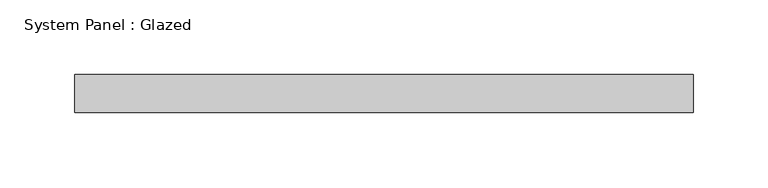
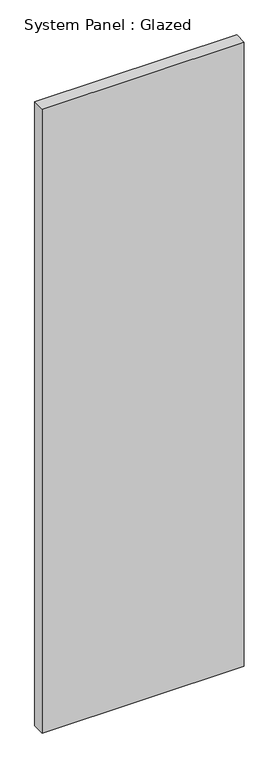
"""IFC4 building model written with IfcOpenShell, lengths in millimetres: plate geometry, System Panel : Glazed."""

from ifc_helpers import new_model, si_unit, origin, origin_with_axes, place, context, project, spatial, polyline, outline, extrude, source, transform, mapped, element, save


def system_panel_glazed_f170b818(model_context):
    return source(origin(), model_context, "Body", "SweptSolid", [
        extrude(outline(polyline([(206.375, 19.05), (-206.375, 19.05), (-206.375, 44.45), (206.375, 44.45), (206.375, 19.05)])), origin_with_axes(), (0.0, 0.0, 1.0), 1345.6043316),
    ])


if __name__ == "__main__":
    model = new_model("IFC4")
    model_context = context("Model", 3, world=origin())
    ifc_project = project(units=[si_unit("LENGTHUNIT", "METRE", prefix="MILLI")], contexts=[model_context])
    site = spatial("IfcSite", under=ifc_project)
    building = spatial("IfcBuilding", under=site)
    placement = place(None, origin())
    system_panel_glazed_shape = system_panel_glazed_f170b818(model_context)
    element("IfcPlate", 1, ObjectType="System Panel : Glazed", at=placement, inside=building, context=model_context, shape_type="MappedRepresentation", body=[
        mapped(system_panel_glazed_shape, transform((0.0, 0.0, 0.0), x_axis=(1.0, 0.0, 0.0), y_axis=(0.0, 1.0, 0.0), z_axis=(0.0, 0.0, 1.0))),
    ])
    save(model, "model.ifc")

# Revit data of these elements
# Type "System Panel : Glazed"
#   Construction Type Id = "GSP4R"
#   Analytic Construction = "1/8 in Pilkington single glazing"
#   Visual Light Transmittance = 0.9
#   Solar Heat Gain Coefficient = 0.86
#   Heat Transfer Coefficient (U) = 1.18115 BTU/(h·ft²·°F)
#   Define Thermal Properties by = 1
# Element 1 (IfcPlate, "System Panel : Glazed")
#   Materials on its faces: "Glass"
# Materials
#   "Glass": class "Glass", colour RGB 0 128 192, transparency 0.75, Description = "Soda Lime Glass", Cost = 0
